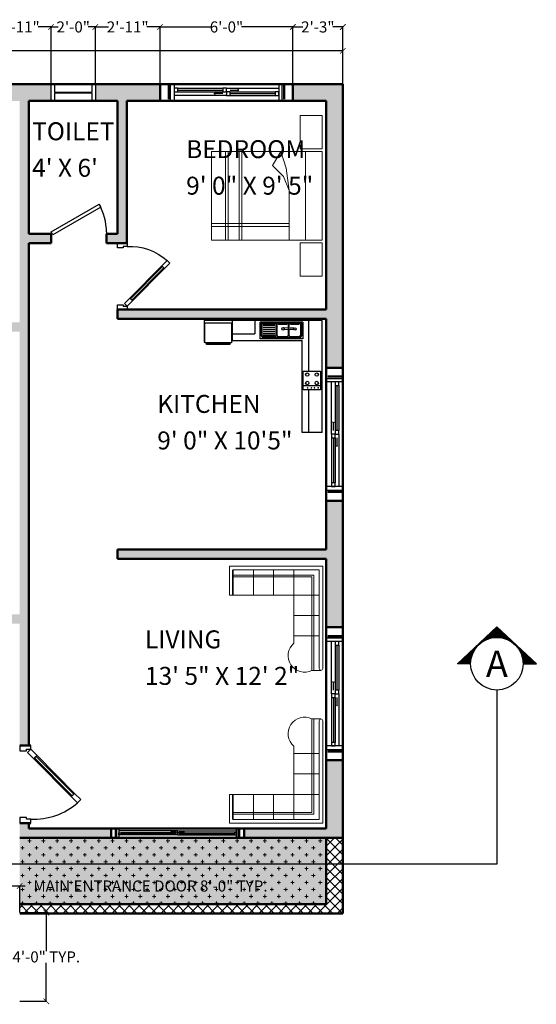
# Model space of a CAD drawing. Units: inches. Extents: x 2278 to 7495, y -71 to 1198.
# Tile 44 of 44: x 7215 to 7495, y 665 to 1198. Entities that reach past the tile are written whole.
import ezdxf
from ezdxf.enums import TextEntityAlignment as Align

# ---------------------------------------------------------------- set-up
doc = ezdxf.new("R2010")
doc.units = ezdxf.units.IN
doc.header["$MEASUREMENT"] = 0
for name, color, linetype, lineweight in [('A-ANNO-DIMS', 2, 'Continuous', 18), ('A-ANNO-SYMB', 1, 'Continuous', 25), ('A-AREA-IDEN', 3, 'Continuous', 18), ('A-Door', 3, 'Continuous', 25), ('A-FLOR-FIXT', 9, 'Continuous', 18), ('A-FURN', 8, 'Continuous', 18), ('A-Glaz', 4, 'Continuous', 25), ('A-Wall', 7, 'Continuous', 50), ('A-WALL-PATT', 8, 'Continuous', 18)]:
    doc.layers.add(name, color=color, linetype=linetype, lineweight=lineweight)
doc.layers.add('TEFRIŞ', color=11, linetype='Continuous')
doc.styles.add('KH-TRUC', font='txt', dxfattribs={"height": 200})
doc.styles.get("Standard").update_dxf_attribs({"font": 'arial.ttf'})
doc.dimstyles.get("Standard").update_dxf_attribs({"dimtxt": 6, "dimasz": 3, "dimexe": 0.18, "dimexo": 0.0625, "dimgap": 0.09, "dimtad": 0, "dimtih": 1, "dimtoh": 1, "dimdec": 0, "dimzin": 0, "dimdsep": 46, "dimlunit": 3, "dimtxsty": 'Standard', "dimblk": 'ARCHTICK', "dimcen": 0.09, "dimadec": 0, "dimazin": 0, "dimtfac": 1, "dimtdec": 0, "dimtofl": 0, "dimtmove": 0, "dimatfit": 3, "dimfxl": 1, "dimtolj": 1, "dimtzin": 0, "dimarcsym": 0})

# ---------------------------------------------------------------- blocks, each defined once
blk = doc.blocks.new('A$C1DF4181C')
blk.add_lwpolyline([(120, 128), (460.7, 466.1), (432.5, 494.5), (91.8, 156.4)], close=True)
blk.add_arc((72.4, 128.7), 593.3, 357.23132, 41.49368)
at = {"layer": 'A-Door'}
for points in [[(517.5, 522.4), (460.7, 466.1), (432.5, 494.5), (489.3, 550.8)], [(35, 100), (0, 100), (0, 0), (50, 0), (50, 50), (50, 60), (35, 60)], [(63.2, 71.6), (120, 128), (91.8, 156.4), (35, 100)], [(665, 100), (665, 60), (650, 60), (650, 50), (650, 0), (700, 0), (700, 100)]]:
    blk.add_lwpolyline(points, close=True, dxfattribs=at)
at = {"layer": 'A-Glaz'}
blk.add_lwpolyline([(112.9, 135.1), (453.6, 473.2), (439.5, 487.4), (98.8, 149.3)], close=True, dxfattribs=at)
at = {"layer": 'A-Wall'}
for p, q in [((0, 0), (0, 100)), ((0, 100), (0, 0)), ((700, 0), (700, 100)), ((700, 0), (700, 100))]:
    blk.add_line(p, q, dxfattribs=at)
blk = doc.blocks.new('*U4')
for p, q in [((0, 0), (0, -6)), ((30, 0), (30, -6))]:
    blk.add_line(p, q)
blk.add_lwpolyline([(0, 0), (25.98, 15), (26.86, 13.48), (0.87, -1.52)], close=True)
blk.add_arc((0, 0), 30, 0, 30)
blk = doc.blocks.new('BED-160')
at = {"color": 0}
for p, q in [((-0.45, 2.35), (-0.45, 2.95)), ((-0.45, 2.95), (-0.05, 2.95)), ((-0.05, 2.95), (-0.05, 2.35)), ((-0.05, 2.35), (-0.45, 2.35)), ((-2.05, 2.3), (-0.05, 2.3)), ((-2.05, 0.7), (-2.05, 2.3)), ((-1.8, 0.7), (-1.8, 2.3)), ((-1.75, 0.7), (-1.75, 2.3)), ((-1.55, 0.7), (-1.55, 2.3)), ((-1.5, 0.7), (-1.5, 2.3)), ((-0.8, 2.3), (-0.95, 2.05)), ((-0.8, 2.3), (-0.7, 2)), ((-0.35, 0.7), (-0.35, 2.3)), ((-0.05, 2.3), (-0.05, 0.7)), ((-0.95, 2.05), (-0.75, 1.85)), ((-0.7, 2), (-0.65, 1.6)), ((-0.75, 1.85), (-0.65, 1.6)), ((-0.65, 1.6), (-0.65, 0.7)), ((-0.65, 1), (-2.05, 1)), ((-0.65, 0.95), (-2.05, 0.95)), ((-0.05, 0.7), (-2.05, 0.7)), ((-0.45, 0.65), (-0.05, 0.65)), ((-0.45, 0.05), (-0.45, 0.65)), ((-0.05, 0.65), (-0.05, 0.05)), ((-0.05, 0.05), (-0.45, 0.05))]:
    blk.add_line(p, q, dxfattribs=at)
blk = doc.blocks.new('A$C008029BD')
at = {"layer": 'TEFRIŞ', "ltscale": 0.05}
for p, q in [((0, 0), (0, -3.55)), ((3.37, 0), (0, 0)), ((3.37, 0), (3.37, -0.6)), ((1.522, -0.4), (0, -0.4)), ((0.05, -0.581), (0.05, -1.869)), ((0.05, -0.581), (0.55, -0.581)), ((0.55, -0.581), (0.55, -1.869)), ((3.37, -0.4), (2.083, -0.4)), ((0.086, -1.773), (0.086, -0.677)), ((0.096, -0.617), (0.454, -0.617)), ((0.099, -0.659), (0.457, -0.659)), ((0.113, -0.954), (0.113, -0.695)), ((0.23, -0.846), (0.229, -0.967)), ((0.28, -0.846), (0.277, -1.158)), ((0.493, -0.695), (0.493, -0.954)), ((0.514, -0.677), (0.514, -1.773)), ((0.6, -2.71), (0.6, -0.6)), ((3.37, -0.6), (0.6, -0.6)), ((0.096, -1.024), (0.454, -1.024)), ((0.457, -0.99), (0.099, -0.99)), ((0.11, -1.319), (0.11, -1.06)), ((0.228, -1.02), (0.227, -1.159)), ((0.49, -1.06), (0.49, -1.319)), ((0.454, -1.355), (0.096, -1.355)), ((0.096, -1.391), (0.454, -1.391)), ((0.11, -1.773), (0.11, -1.427)), ((0.154, -1.773), (0.154, -1.427)), ((0.214, -1.773), (0.214, -1.427)), ((0.274, -1.773), (0.274, -1.427)), ((0.334, -1.773), (0.334, -1.427)), ((0.39, -1.773), (0.39, -1.427)), ((0.444, -1.773), (0.444, -1.427)), ((0.49, -1.427), (0.49, -1.773)), ((0, -2.025), (0.4, -2.025)), ((0.55, -1.869), (0.05, -1.869)), ((0.454, -1.809), (0.096, -1.809)), ((0.454, -1.833), (0.096, -1.833)), ((0.4, -2.71), (0.4, -2.025)), ((0, -2.71), (0.6, -2.71)), ((0, -3.55), (0.65, -3.55))]:
    blk.add_line(p, q, dxfattribs=at)
at = {"layer": 'TEFRIŞ'}
blk.add_line((1.969, -0.05), (1.969, -0.572), dxfattribs=at)
at = {"layer": 'TEFRIŞ', "ltscale": 0.05}
for points in [[(1.522, -0.05), (2.083, -0.05), (2.083, -0.572), (1.522, -0.572)], [(0.67, -2.73), (0.67, -3.53), (0.07, -3.53), (0.07, -2.73)], [(0.72, -2.78), (0.72, -3.48), (0.67, -3.48), (0.67, -2.78)]]:
    blk.add_lwpolyline(points, close=True, dxfattribs=at)
at = {"layer": 'TEFRIŞ', "const_width": 0.025}
for points in [[(2.014, -0.123, 1), (2.039, -0.123, 1)], [(2.014, -0.236, 1), (2.039, -0.236, 1)], [(2.014, -0.327, 1), (2.039, -0.327, 1)], [(2.014, -0.44, 1), (2.039, -0.44, 1)]]:
    blk.add_lwpolyline(points, format="xyb", close=True, dxfattribs=at)
at = {"layer": 'TEFRIŞ', "ltscale": 0.05}
for centre, radius in [((1.628, -0.164), 0.0505), ((1.628, -0.45), 0.0505), ((0.255, -0.82), 0.036), ((0.252, -1.184), 0.036)]:
    blk.add_circle(centre, radius, dxfattribs=at)
at = {"layer": 'TEFRIŞ'}
for centre in [(1.88, -0.164), (1.88, -0.45)]:
    blk.add_circle(centre, 0.0505, dxfattribs=at)
at = {"layer": 'TEFRIŞ', "ltscale": 0.05}
for centre, radius, start, end in [((0.108, -0.649), 0.0351, 110.4976, 230.5777), ((0.118, -0.673), 0.023, 143.9853, 258.5157), ((0.454, -0.677), 0.06, 0, 90), ((0.457, -0.695), 0.036, 0, 90), ((0.115, -1.038), 0.023, 143.9853, 258.5157), ((0.118, -0.976), 0.023, 101.4843, 216.0147), ((0.454, -1.06), 0.036, 0, 90), ((0.457, -0.954), 0.036, 270, 0), ((0.115, -1.341), 0.023, 101.4843, 216.0147), ((0.115, -1.405), 0.023, 143.9853, 258.5157), ((0.454, -1.319), 0.036, 270, 0), ((0.454, -1.427), 0.036, 0, 90), ((0.108, -1.801), 0.0351, 129.4223, 249.5024), ((0.115, -1.796), 0.023, 101.4843, 216.0147), ((0.454, -1.773), 0.06, 270, 0), ((0.454, -1.773), 0.036, 270, 0)]:
    blk.add_arc(centre, radius, start, end, dxfattribs=at)
blk = doc.blocks.new('_ArchTick')
at = {"color": 0, "linetype": 'ByBlock', "const_width": 0.15}
blk.add_lwpolyline([(-0.5, -0.5), (0.5, 0.5)], dxfattribs=at)
blk = doc.blocks.new('*D28')
at = {"layer": 'A-ANNO-DIMS', "color": 0, "lineweight": -2, "transparency": 16777216}
for p, q in [((6987.12, 1163.53), (6987.12, 1181.72)), ((6987.12, 1181.54), (7178.22, 1181.54)), ((7390.12, 1181.54), (7199.01, 1181.54)), ((7390.12, 1163.53), (7390.12, 1181.72))]:
    blk.add_line(p, q, dxfattribs=at)
at = {"layer": 'Defpoints', "color": 0, "transparency": 16777216}
for p in [(7390.12, 1181.54), (6987.12, 1163.47), (7390.12, 1163.47)]:
    blk.add_point(p, dxfattribs=at)
at = {"layer": 'A-ANNO-DIMS', "color": 0, "lineweight": -2, "transparency": 16777216, "xscale": 3, "yscale": 3, "zscale": 3, "rotation": 180}
blk.add_blockref('_ArchTick', (6987.12, 1181.54), dxfattribs=at)
at = {"layer": 'A-ANNO-DIMS', "color": 0, "lineweight": -2, "transparency": 16777216, "xscale": 3, "yscale": 3, "zscale": 3}
blk.add_blockref('_ArchTick', (7390.12, 1181.54), dxfattribs=at)
at = {"layer": 'A-ANNO-DIMS', "color": 0, "transparency": 16777216, "insert": (7188.62, 1181.54), "char_height": 6, "attachment_point": 5}
blk.add_mtext('\\A1;33\'-7"', dxfattribs=at)
blk = doc.blocks.new('*X31')
at = {"color": 0}
for p, q in [((19.68, 20.47), (19.71, 20.51)), ((19.68, 20.38), (19.76, 20.46)), ((19.68, 20.29), (19.8, 20.42)), ((19.68, 20.21), (19.84, 20.37)), ((19.68, 20.12), (19.88, 20.33)), ((19.68, 20.03), (19.93, 20.28)), ((19.68, 19.94), (19.97, 20.23)), ((19.68, 19.85), (20.01, 20.19)), ((19.68, 19.76), (20.05, 20.14)), ((19.68, 19.68), (20.1, 20.1)), ((19.68, 19.59), (20.14, 20.05)), ((19.68, 19.5), (20.18, 20.01)), ((19.68, 19.41), (20.22, 19.96)), ((19.68, 19.32), (20.27, 19.91)), ((19.68, 19.23), (20.31, 19.87)), ((19.68, 19.15), (20.35, 19.82)), ((19.68, 19.06), (20.4, 19.78)), ((19.68, 18.97), (20.44, 19.73)), ((19.68, 18.88), (20.48, 19.69)), ((19.68, 18.79), (20.52, 19.64)), ((19.68, 18.7), (20.57, 19.59)), ((19.68, 18.62), (20.61, 19.55)), ((19.68, 18.53), (20.65, 19.5)), ((19.68, 18.44), (20.69, 19.46)), ((19.68, 18.35), (20.74, 19.41)), ((19.68, 18.26), (20.78, 19.37)), ((19.68, 18.17), (20.82, 19.32)), ((19.68, 18.08), (20.86, 19.27)), ((19.73, 18.05), (20.91, 19.23)), ((19.81, 18.05), (20.95, 19.18)), ((19.9, 18.04), (20.99, 19.14)), ((19.98, 18.04), (21.04, 19.09)), ((20.06, 18.03), (21.08, 19.05)), ((20.15, 18.03), (21.12, 19)), ((20.23, 18.02), (21.16, 18.95)), ((20.31, 18.01), (21.21, 18.91)), ((20.38, 18), (21.25, 18.86)), ((20.46, 17.99), (21.29, 18.82)), ((20.54, 17.97), (21.33, 18.77)), ((20.61, 17.96), (21.38, 18.73)), ((20.68, 17.94), (21.42, 18.68)), ((20.76, 17.93), (21.46, 18.63)), ((20.83, 17.91), (21.5, 18.59)), ((20.9, 17.9), (21.55, 18.54)), ((20.97, 17.88), (21.59, 18.5)), ((21.04, 17.86), (21.63, 18.45)), ((21.11, 17.84), (21.68, 18.41)), ((21.18, 17.82), (21.72, 18.36)), ((21.24, 17.8), (21.76, 18.31)), ((21.31, 17.77), (21.8, 18.27)), ((21.37, 17.75), (21.85, 18.22)), ((21.44, 17.73), (21.89, 18.18)), ((21.5, 17.7), (21.93, 18.13)), ((21.57, 17.68), (21.97, 18.08)), ((21.63, 17.65), (22.02, 18.04)), ((21.69, 17.62), (22.06, 17.99)), ((21.75, 17.6), (22.1, 17.95)), ((21.81, 17.57), (22.14, 17.9)), ((21.87, 17.54), (22.19, 17.86)), ((21.93, 17.51), (22.23, 17.81)), ((21.99, 17.48), (22.27, 17.76)), ((22.05, 17.45), (22.32, 17.72)), ((22.1, 17.42), (22.36, 17.67)), ((22.16, 17.39), (22.4, 17.63)), ((22.22, 17.35), (22.44, 17.58)), ((22.27, 17.32), (22.49, 17.54)), ((22.33, 17.29), (22.53, 17.49)), ((22.38, 17.25), (22.57, 17.44)), ((22.43, 17.22), (22.61, 17.4)), ((22.49, 17.18), (22.66, 17.35)), ((22.54, 17.15), (22.7, 17.31)), ((22.59, 17.11), (22.74, 17.26)), ((22.64, 17.07), (22.78, 17.22)), ((22.69, 17.04), (22.83, 17.17)), ((22.74, 17), (22.87, 17.12)), ((22.79, 16.96), (22.91, 17.08)), ((22.84, 16.92), (22.96, 17.03)), ((22.89, 16.88), (23, 16.99)), ((22.94, 16.84), (23.04, 16.94)), ((22.98, 16.8), (23.08, 16.9)), ((23.03, 16.75), (23.13, 16.85)), ((23.08, 16.71), (23.17, 16.8)), ((23.12, 16.67), (23.21, 16.76)), ((23.17, 16.63), (23.25, 16.71)), ((23.21, 16.58), (23.3, 16.67)), ((23.26, 16.54), (23.34, 16.62)), ((23.3, 16.49), (23.38, 16.58)), ((23.34, 16.45), (23.42, 16.53)), ((23.38, 16.4), (23.47, 16.48)), ((23.43, 16.35), (23.51, 16.44)), ((23.47, 16.31), (23.55, 16.39)), ((23.51, 16.26), (23.6, 16.35)), ((23.55, 16.21), (23.64, 16.3)), ((23.59, 16.16), (23.68, 16.26)), ((23.63, 16.11), (23.72, 16.21)), ((23.66, 16.06), (23.77, 16.16)), ((23.7, 16.01), (23.81, 16.12)), ((23.74, 15.96), (23.85, 16.07)), ((23.78, 15.91), (23.89, 16.03)), ((23.81, 15.86), (23.94, 15.98)), ((23.85, 15.8), (23.98, 15.94)), ((23.88, 15.75), (24.02, 15.89)), ((23.92, 15.7), (24.06, 15.84)), ((23.95, 15.64), (24.11, 15.8)), ((23.98, 15.59), (24.15, 15.75)), ((24.02, 15.53), (24.19, 15.71)), ((24.05, 15.47), (24.24, 15.66)), ((24.08, 15.42), (24.28, 15.62)), ((24.11, 15.36), (24.32, 15.57)), ((24.14, 15.3), (24.36, 15.52)), ((24.17, 15.24), (24.41, 15.48)), ((24.2, 15.18), (24.45, 15.43)), ((24.23, 15.12), (24.49, 15.39)), ((24.25, 15.06), (24.53, 15.34)), ((24.28, 15), (24.58, 15.3)), ((24.31, 14.94), (24.62, 15.25)), ((24.33, 14.87), (24.66, 15.2)), ((24.36, 14.81), (24.7, 15.16)), ((24.38, 14.74), (24.75, 15.11)), ((24.4, 14.68), (24.79, 15.07)), ((24.42, 14.61), (24.83, 15.02)), ((24.45, 14.55), (24.88, 14.98)), ((24.04, 10.6), (26.58, 13.15)), ((24.14, 10.79), (26.54, 13.19)), ((24.22, 10.96), (26.5, 13.24)), ((24.29, 11.12), (26.45, 13.28)), ((24.35, 11.27), (26.41, 13.33)), ((24.4, 11.41), (26.37, 13.38)), ((24.44, 11.54), (26.33, 13.42)), ((24.47, 14.48), (24.92, 14.93)), ((24.48, 11.66), (26.28, 13.47)), ((24.49, 14.41), (24.96, 14.88)), ((24.51, 14.34), (25, 14.84)), ((24.51, 11.79), (26.24, 13.51)), ((24.52, 14.27), (25.05, 14.79)), ((24.54, 14.2), (25.09, 14.75)), ((24.54, 11.9), (26.2, 13.56)), ((24.56, 14.13), (25.13, 14.7)), ((24.57, 14.06), (25.17, 14.66)), ((24.57, 12.02), (26.16, 13.6)), ((24.59, 13.98), (25.22, 14.61)), ((24.59, 12.13), (26.11, 13.65)), ((24.6, 13.91), (25.26, 14.56)), ((24.61, 13.83), (25.3, 14.52)), ((24.61, 12.24), (26.07, 13.7)), ((24.63, 13.75), (25.35, 14.47)), ((24.63, 12.34), (26.03, 13.74)), ((24.64, 13.68), (25.39, 14.43)), ((24.64, 12.44), (25.99, 13.79)), ((24.65, 13.6), (25.43, 14.38)), ((24.65, 13.52), (25.47, 14.34)), ((24.65, 12.54), (25.94, 13.83)), ((24.66, 13.44), (25.52, 14.29)), ((24.66, 12.64), (25.9, 13.88)), ((24.67, 13.35), (25.56, 14.24)), ((24.67, 13.27), (25.6, 14.2)), ((24.67, 13.18), (25.64, 14.15)), ((24.67, 12.92), (25.77, 14.02)), ((24.67, 12.83), (25.81, 13.97)), ((24.67, 12.73), (25.86, 13.92)), ((24.68, 13.1), (25.69, 14.11)), ((24.68, 13.01), (25.73, 14.06)), ((19.68, 5.98), (25.68, 11.98)), ((23.72, 10.11), (26.67, 13.06)), ((23.91, 10.38), (26.63, 13.1)), ((19.68, 5.89), (24.44, 10.65)), ((19.68, 5.8), (23.2, 9.32)), ((19.68, 6.06), (22.61, 9)), ((19.68, 6.15), (22.34, 8.81)), ((19.68, 6.24), (22.12, 8.69)), ((19.68, 6.33), (21.93, 8.58)), ((19.68, 6.42), (21.76, 8.5)), ((19.68, 6.51), (21.6, 8.43)), ((19.68, 6.59), (21.46, 8.37)), ((19.68, 6.68), (21.32, 8.32)), ((19.68, 6.77), (21.19, 8.28)), ((19.68, 6.86), (21.06, 8.24)), ((19.68, 6.95), (20.94, 8.21)), ((19.68, 7.04), (20.82, 8.18)), ((19.68, 7.12), (20.71, 8.15)), ((19.68, 7.21), (20.6, 8.13)), ((19.68, 7.3), (20.49, 8.11)), ((19.68, 7.39), (20.38, 8.1)), ((19.68, 7.48), (20.28, 8.08)), ((19.68, 7.57), (20.18, 8.07)), ((19.68, 7.74), (19.99, 8.06)), ((19.68, 7.66), (20.08, 8.06)), ((19.68, 8.01), (19.71, 8.05)), ((19.68, 7.92), (19.8, 8.05)), ((19.68, 7.83), (19.9, 8.05)), ((19.68, 5.71), (21.96, 8)), ((19.68, 5.62), (20.73, 6.67))]:
    blk.add_line(p, q, dxfattribs=at)
blk = doc.blocks.new('A$C695C76AC')
for p, q in [((5.36, 5), (12.86, 12)), ((20.36, 5), (12.86, 12)), ((7.86, 5), (5.36, 5)), ((17.86, 5), (20.36, 5))]:
    blk.add_line(p, q)
blk.add_circle((12.86, 5), 5)
at = {"rotation": 90}
blk.add_blockref('*X31', (25.9, -14.68), dxfattribs=at)
at = {"style": 'KH-TRUC'}
blk.add_attdef('KH-MC', text='', height=5, dxfattribs=at).set_placement((12.86, 5), align=Align.MIDDLE_CENTER)
blk = doc.blocks.new('*D55')
at = {"layer": 'A-ANNO-DIMS', "color": 0, "lineweight": -2, "transparency": 16777216}
for p, q in [((7119.12, 715.03), (7119.12, 729.55)), ((7119.12, 729.37), (7215.12, 729.37)), ((7215.12, 715.03), (7215.12, 729.55)), ((7215.12, 729.37), (7218.12, 729.37))]:
    blk.add_line(p, q, dxfattribs=at)
at = {"layer": 'Defpoints', "color": 0, "transparency": 16777216}
for p in [(7215.12, 729.37), (7119.12, 714.97), (7215.12, 714.97)]:
    blk.add_point(p, dxfattribs=at)
at = {"layer": 'A-ANNO-DIMS', "color": 0, "lineweight": -2, "transparency": 16777216, "xscale": 3, "yscale": 3, "zscale": 3, "rotation": 180}
blk.add_blockref('_ArchTick', (7119.12, 729.37), dxfattribs=at)
at = {"layer": 'A-ANNO-DIMS', "color": 0, "lineweight": -2, "transparency": 16777216, "xscale": 3, "yscale": 3, "zscale": 3}
blk.add_blockref('_ArchTick', (7215.12, 729.37), dxfattribs=at)
at = {"layer": 'A-ANNO-DIMS', "color": 0, "transparency": 16777216, "insert": (7285.95, 729.37), "char_height": 6, "attachment_point": 5}
blk.add_mtext('\\A1;MAIN ENTRANCE DOOR 8\'-0" TYP.', dxfattribs=at)
blk = doc.blocks.new('*D56')
at = {"layer": 'A-ANNO-DIMS', "color": 0, "lineweight": -2, "transparency": 16777216}
for p, q in [((7215.18, 714.97), (7229.7, 714.97)), ((7229.52, 714.97), (7229.52, 694.12)), ((7229.52, 666.97), (7229.52, 687.81)), ((7215.18, 666.97), (7229.7, 666.97))]:
    blk.add_line(p, q, dxfattribs=at)
at = {"layer": 'Defpoints', "color": 0, "transparency": 16777216}
for p in [(7215.12, 714.97), (7215.12, 666.97), (7229.52, 666.97)]:
    blk.add_point(p, dxfattribs=at)
at = {"layer": 'A-ANNO-DIMS', "color": 0, "lineweight": -2, "transparency": 16777216, "xscale": 3, "yscale": 3, "zscale": 3}
for p, rotation in [((7229.52, 714.97), 90), ((7229.52, 666.97), 270)]:
    blk.add_blockref('_ArchTick', p, dxfattribs=dict(at, rotation=rotation))
at = {"layer": 'A-ANNO-DIMS', "color": 0, "transparency": 16777216, "insert": (7229.52, 690.97), "char_height": 6, "attachment_point": 5}
blk.add_mtext('\\A1;4\'-0" TYP.', dxfattribs=at)
blk = doc.blocks.new('*D97')
at = {"layer": 'A-ANNO-DIMS', "color": 0, "lineweight": -2, "transparency": 16777216}
for p, q in [((7197.12, 1163.53), (7197.12, 1194.65)), ((7197.12, 1194.47), (7204.17, 1194.47)), ((7232.12, 1194.47), (7225.06, 1194.47)), ((7232.12, 1163.53), (7232.12, 1194.65))]:
    blk.add_line(p, q, dxfattribs=at)
at = {"layer": 'Defpoints', "color": 0, "transparency": 16777216}
for p in [(7232.12, 1194.47), (7197.12, 1163.47), (7232.12, 1163.47)]:
    blk.add_point(p, dxfattribs=at)
at = {"layer": 'A-ANNO-DIMS', "color": 0, "lineweight": -2, "transparency": 16777216, "xscale": 3, "yscale": 3, "zscale": 3, "rotation": 180}
blk.add_blockref('_ArchTick', (7197.12, 1194.47), dxfattribs=at)
at = {"layer": 'A-ANNO-DIMS', "color": 0, "lineweight": -2, "transparency": 16777216, "xscale": 3, "yscale": 3, "zscale": 3}
blk.add_blockref('_ArchTick', (7232.12, 1194.47), dxfattribs=at)
at = {"layer": 'A-ANNO-DIMS', "color": 0, "transparency": 16777216, "insert": (7214.62, 1194.47), "char_height": 6, "attachment_point": 5}
blk.add_mtext('\\A1;2\'-11"', dxfattribs=at)
blk = doc.blocks.new('*D98')
at = {"layer": 'A-ANNO-DIMS', "color": 0, "lineweight": -2, "transparency": 16777216}
for p, q in [((7232.12, 1163.53), (7232.12, 1194.65)), ((7232.12, 1194.47), (7236, 1194.47)), ((7256.12, 1194.47), (7252.23, 1194.47)), ((7256.12, 1163.53), (7256.12, 1194.65))]:
    blk.add_line(p, q, dxfattribs=at)
at = {"layer": 'Defpoints', "color": 0, "transparency": 16777216}
for p in [(7256.12, 1194.47), (7232.12, 1163.47), (7256.12, 1163.47)]:
    blk.add_point(p, dxfattribs=at)
at = {"layer": 'A-ANNO-DIMS', "color": 0, "lineweight": -2, "transparency": 16777216, "xscale": 3, "yscale": 3, "zscale": 3, "rotation": 180}
blk.add_blockref('_ArchTick', (7232.12, 1194.47), dxfattribs=at)
at = {"layer": 'A-ANNO-DIMS', "color": 0, "lineweight": -2, "transparency": 16777216, "xscale": 3, "yscale": 3, "zscale": 3}
blk.add_blockref('_ArchTick', (7256.12, 1194.47), dxfattribs=at)
at = {"layer": 'A-ANNO-DIMS', "color": 0, "transparency": 16777216, "insert": (7244.12, 1194.47), "char_height": 6, "attachment_point": 5}
blk.add_mtext('\\A1;2\'-0"', dxfattribs=at)
blk = doc.blocks.new('*D99')
at = {"layer": 'A-ANNO-DIMS', "color": 0, "lineweight": -2, "transparency": 16777216}
for p, q in [((7256.12, 1163.53), (7256.12, 1194.65)), ((7256.12, 1194.47), (7263.17, 1194.47)), ((7291.12, 1194.47), (7284.06, 1194.47)), ((7291.12, 1163.53), (7291.12, 1194.65))]:
    blk.add_line(p, q, dxfattribs=at)
at = {"layer": 'Defpoints', "color": 0, "transparency": 16777216}
for p in [(7291.12, 1194.47), (7256.12, 1163.47), (7291.12, 1163.47)]:
    blk.add_point(p, dxfattribs=at)
at = {"layer": 'A-ANNO-DIMS', "color": 0, "lineweight": -2, "transparency": 16777216, "xscale": 3, "yscale": 3, "zscale": 3, "rotation": 180}
blk.add_blockref('_ArchTick', (7256.12, 1194.47), dxfattribs=at)
at = {"layer": 'A-ANNO-DIMS', "color": 0, "lineweight": -2, "transparency": 16777216, "xscale": 3, "yscale": 3, "zscale": 3}
blk.add_blockref('_ArchTick', (7291.12, 1194.47), dxfattribs=at)
at = {"layer": 'A-ANNO-DIMS', "color": 0, "transparency": 16777216, "insert": (7273.62, 1194.47), "char_height": 6, "attachment_point": 5}
blk.add_mtext('\\A1;2\'-11"', dxfattribs=at)
blk = doc.blocks.new('*D100')
at = {"layer": 'A-ANNO-DIMS', "color": 0, "lineweight": -2, "transparency": 16777216}
for p, q in [((7291.12, 1163.53), (7291.12, 1194.65)), ((7291.12, 1194.47), (7319.03, 1194.47)), ((7363.12, 1194.47), (7335.2, 1194.47)), ((7363.12, 1163.53), (7363.12, 1194.65))]:
    blk.add_line(p, q, dxfattribs=at)
at = {"layer": 'Defpoints', "color": 0, "transparency": 16777216}
for p in [(7363.12, 1194.47), (7291.12, 1163.47), (7363.12, 1163.47)]:
    blk.add_point(p, dxfattribs=at)
at = {"layer": 'A-ANNO-DIMS', "color": 0, "lineweight": -2, "transparency": 16777216, "xscale": 3, "yscale": 3, "zscale": 3, "rotation": 180}
blk.add_blockref('_ArchTick', (7291.12, 1194.47), dxfattribs=at)
at = {"layer": 'A-ANNO-DIMS', "color": 0, "lineweight": -2, "transparency": 16777216, "xscale": 3, "yscale": 3, "zscale": 3}
blk.add_blockref('_ArchTick', (7363.12, 1194.47), dxfattribs=at)
at = {"layer": 'A-ANNO-DIMS', "color": 0, "transparency": 16777216, "insert": (7327.12, 1194.47), "char_height": 6, "attachment_point": 5}
blk.add_mtext('\\A1;6\'-0"', dxfattribs=at)
blk = doc.blocks.new('*D101')
at = {"layer": 'A-ANNO-DIMS', "color": 0, "lineweight": -2, "transparency": 16777216}
for p, q in [((7363.12, 1163.53), (7363.12, 1194.65)), ((7363.12, 1194.47), (7368.5, 1194.47)), ((7390.12, 1194.47), (7384.73, 1194.47)), ((7390.12, 1163.53), (7390.12, 1194.65))]:
    blk.add_line(p, q, dxfattribs=at)
at = {"layer": 'Defpoints', "color": 0, "transparency": 16777216}
for p in [(7390.12, 1194.47), (7363.12, 1163.47), (7390.12, 1163.47)]:
    blk.add_point(p, dxfattribs=at)
at = {"layer": 'A-ANNO-DIMS', "color": 0, "lineweight": -2, "transparency": 16777216, "xscale": 3, "yscale": 3, "zscale": 3, "rotation": 180}
blk.add_blockref('_ArchTick', (7363.12, 1194.47), dxfattribs=at)
at = {"layer": 'A-ANNO-DIMS', "color": 0, "lineweight": -2, "transparency": 16777216, "xscale": 3, "yscale": 3, "zscale": 3}
blk.add_blockref('_ArchTick', (7390.12, 1194.47), dxfattribs=at)
at = {"layer": 'A-ANNO-DIMS', "color": 0, "transparency": 16777216, "insert": (7376.62, 1194.47), "char_height": 6, "attachment_point": 5}
blk.add_mtext('\\A1;2\'-3"', dxfattribs=at)

msp = doc.modelspace()

# ---------------------------------------------------------------- hatches: boundary and pattern name
at = {"layer": 'A-WALL-PATT'}
h = msp.add_hatch(dxfattribs=at)
h.set_pattern_fill('ANSI36', color=256, scale=30)
h.set_pattern_definition([(45, (4673.2453, 0), (1.988738, 7.2920387), [9.375, -1.875, 0, -1.875])])
h.paths.add_polyline_path([(7016.37, 957.47), (6996.12, 957.47), (6996.12, 1029.47), (7025.12, 1029.47), (7025.12, 1034.47), (6996.12, 1034.47), (6996.12, 1154.47), (7013.12, 1154.47), (7013.12, 1163.47), (6987.12, 1163.47), (6987.12, 710.47), (7119.12, 710.47), (7119.12, 719.47), (6996.12, 719.47), (6996.12, 807.47), (7078.12, 807.47), (7078.12, 812.47), (7066.12, 812.47), (7066.12, 881.47), (7061.12, 881.47), (7061.12, 812.47), (6996.12, 812.47), (6996.12, 911.47), (7019.12, 911.47), (7019.12, 916.47), (6996.12, 916.47), (6996.12, 952.47), (7016.37, 952.47)])
h.paths.add_polyline_path([(7125.12, 1163.47), (7085.12, 1163.47), (7085.12, 1154.47), (7102.12, 1154.47), (7102.12, 1034.47), (7102.12, 1029.47), (7107.12, 1029.47), (7107.12, 1154.47), (7125.12, 1154.47)])
h.paths.add_polyline_path([(7232.12, 1163.47), (7197.12, 1163.47), (7197.12, 1154.47), (7215.12, 1154.47), (7215.12, 1034.47), (7149.12, 1034.47), (7149.12, 1029.47), (7215.12, 1029.47), (7215.12, 943.47), (7215.12, 940.13), (7215.12, 876.47), (7167.12, 876.47), (7167.12, 943.47), (7162.12, 943.47), (7162.12, 871.47), (7162.12, 865.74), (7167.12, 865.74), (7167.12, 871.47), (7215.12, 871.47), (7215.12, 805.47), (7220.12, 805.47), (7220.12, 1077.47), (7232.12, 1077.47), (7232.12, 1082.47), (7220.12, 1082.47), (7220.12, 1154.47), (7232.12, 1154.47)])
h.paths.add_polyline_path([(7390.12, 937.97), (7381.12, 937.97), (7381.12, 911.47), (7268.12, 911.47), (7268.12, 906.47), (7381.12, 906.47), (7381.12, 869.47), (7390.12, 869.47)])
h.paths.add_polyline_path([(7390.12, 1163.47), (7363.12, 1163.47), (7363.12, 1154.47), (7381.12, 1154.47), (7381.12, 1041.47), (7268.12, 1041.47), (7268.12, 1036.47), (7381.12, 1036.47), (7381.12, 1009.97), (7390.12, 1009.97)])
h.paths.add_polyline_path([(7291.12, 1163.47), (7256.12, 1163.47), (7256.12, 1154.47), (7268.12, 1154.47), (7268.12, 1082.47), (7262.12, 1082.47), (7262.12, 1077.47), (7273.12, 1077.47), (7273.12, 1154.47), (7291.12, 1154.47)])
h.paths.add_polyline_path([(7390.12, 797.47), (7381.12, 797.47), (7381.12, 760.47), (7336.62, 760.47), (7336.62, 755.47), (7390.12, 755.47)])
h.paths.add_polyline_path([(7264.62, 760.47), (7220.12, 760.47), (7220.12, 763.47), (7215.12, 763.47), (7215.12, 755.47), (7264.62, 755.47)])
h = msp.add_hatch(dxfattribs=at)
h.set_pattern_fill('ANSI37', color=256, scale=30)
h.set_pattern_definition([(45, (4673.2453, 0), (-2.6516504, 2.6516504), []), (135, (4673.2453, 0), (-2.6516504, -2.6516504), [])])
h.paths.add_polyline_path([(7390.12, 755.47), (7381.12, 755.47), (7381.12, 719.47), (7215.12, 719.47), (7215.12, 714.47), (7390.12, 714.47)])
at = {"layer": 'A-WALL-PATT', "transparency": 33554562}
h = msp.add_hatch(color=256, dxfattribs=at)
h.dxf.hatch_style = 1
h.paths.add_polyline_path([(7381.12, 755.47), (7215.12, 755.47), (7215.12, 719.47), (7381.12, 719.47)])
h = msp.add_hatch(dxfattribs=at)
h.set_pattern_fill('CROSS', color=256, scale=15)
h.set_pattern_definition([(0, (4673.2453, 0), (3.75, 3.75), [1.875, -5.625]), (90, (4674.1828, -0.9375), (-3.75, 3.75), [1.875, -5.625])])
h.paths.add_polyline_path([(7381.12, 755.47), (7215.12, 755.47), (7215.12, 719.47), (7381.12, 719.47)])

# ---------------------------------------------------------------- linework, layer by layer
at = {"layer": 'A-ANNO-SYMB'}
for p, q in [((7473.67, 741.41), (7473.67, 835.33)), ((6942.63, 741.41), (7473.67, 741.41))]:
    msp.add_line(p, q, dxfattribs=at)
at = {"layer": 'A-FURN'}
for p, q in [((7379.26, 902.55), (7328.74, 902.55)), ((7328.74, 902.55), (7328.74, 886.91)), ((7379.26, 847.04), (7379.26, 902.55)), ((7330.37, 900.59), (7330.37, 886.91)), ((7377.31, 900.59), (7330.7, 900.59)), ((7330.7, 900.59), (7330.7, 886.91)), ((7374.37, 897.66), (7330.7, 897.66)), ((7373.4, 896.68), (7330.7, 896.68)), ((7341.78, 900.59), (7341.78, 886.91)), ((7352.54, 900.59), (7352.54, 886.91)), ((7363.62, 900.59), (7363.62, 864.74)), ((7373.4, 846.06), (7373.4, 896.68)), ((7374.37, 846.06), (7374.37, 897.66)), ((7377.31, 847.04), (7377.31, 900.59)), ((7328.74, 886.91), (7377.31, 886.91)), ((7363.62, 889.51), (7363.62, 864.74)), ((7363.62, 875.82), (7377.31, 875.82)), ((7363.62, 864.74), (7377.31, 864.74)), ((7363.62, 864.74), (7377.31, 864.74)), ((7363.62, 864.74), (7363.62, 860.83)), ((7378.29, 846.06), (7373.4, 846.06)), ((7373.4, 819.82), (7373.4, 769.19)), ((7378.29, 819.82), (7373.4, 819.82)), ((7374.37, 819.82), (7374.37, 768.22)), ((7377.31, 818.84), (7377.31, 765.28)), ((7379.26, 818.84), (7379.26, 763.33)), ((7363.62, 801.14), (7363.62, 805.05)), ((7363.62, 765.28), (7363.62, 801.14)), ((7363.62, 776.37), (7363.62, 801.14)), ((7363.62, 801.14), (7377.31, 801.14)), ((7363.62, 801.14), (7377.31, 801.14)), ((7363.62, 790.05), (7377.31, 790.05)), ((7328.74, 778.97), (7377.31, 778.97)), ((7328.74, 763.33), (7328.74, 778.97)), ((7330.37, 765.28), (7330.37, 778.97)), ((7330.7, 765.28), (7330.7, 778.97)), ((7341.78, 765.28), (7341.78, 778.97)), ((7352.54, 765.28), (7352.54, 778.97)), ((7373.4, 769.19), (7330.7, 769.19)), ((7374.37, 768.22), (7330.7, 768.22)), ((7379.26, 763.33), (7328.74, 763.33)), ((7377.31, 765.28), (7330.7, 765.28))]:
    msp.add_line(p, q, dxfattribs=at)
for centre, radius, start, end in [((7369.43, 854.05), 8.93, 130.6021, 296.4078), ((7378.29, 847.04), 0.978, 180, 0), ((7369.43, 811.82), 8.93, 63.5922, 229.3979), ((7378.29, 818.84), 0.978, 0, 180)]:
    msp.add_arc(centre, radius, start, end, dxfattribs=at)
at = {"layer": 'A-Glaz'}
for p, q in [((7232.12, 1163.47), (7256.12, 1163.47)), ((7232.12, 1154.47), (7232.12, 1163.47)), ((7234.12, 1159.17), (7234.12, 1163.47)), ((7254.12, 1163.47), (7254.12, 1159.17)), ((7256.12, 1163.47), (7256.12, 1154.47)), ((7298.82, 1163.47), (7355.41, 1163.47)), ((7234.12, 1159.17), (7254.12, 1159.17)), ((7234.12, 1154.47), (7234.12, 1158.77)), ((7234.12, 1158.77), (7254.12, 1158.77)), ((7254.12, 1158.77), (7254.12, 1154.47)), ((7327.12, 1157.39), (7298.82, 1157.39)), ((7300.77, 1161.3), (7325.16, 1161.3)), ((7300.77, 1160.32), (7325.16, 1160.32)), ((7300.77, 1159.35), (7325.16, 1159.35)), ((7325.16, 1158.37), (7320.97, 1158.37)), ((7327.12, 1161.3), (7355.41, 1161.3)), ((7329.07, 1160.32), (7333.26, 1160.32)), ((7329.07, 1159.35), (7353.46, 1159.35)), ((7329.07, 1158.37), (7353.46, 1158.37)), ((7329.07, 1157.39), (7353.46, 1157.39)), ((7256.12, 1154.47), (7232.12, 1154.47)), ((7298.82, 1154.47), (7355.41, 1154.47)), ((7381.12, 1002.27), (7381.12, 945.67)), ((7384.04, 973.97), (7384.04, 1002.27)), ((7390.12, 1002.27), (7390.12, 945.67)), ((7385.99, 1000.31), (7385.99, 975.92)), ((7386.97, 1000.31), (7386.97, 975.92)), ((7387.95, 1000.31), (7387.95, 975.92)), ((7385.02, 975.92), (7385.02, 980.11)), ((7384.04, 972.01), (7384.04, 947.62)), ((7385.02, 972.01), (7385.02, 947.62)), ((7385.99, 972.01), (7385.99, 947.62)), ((7386.97, 972.01), (7386.97, 967.82)), ((7387.95, 973.97), (7387.95, 945.67)), ((7381.12, 861.77), (7381.12, 805.17)), ((7384.04, 833.47), (7384.04, 861.77)), ((7385.99, 859.81), (7385.99, 835.42)), ((7386.97, 859.81), (7386.97, 835.42)), ((7387.95, 859.81), (7387.95, 835.42)), ((7390.12, 861.77), (7390.12, 805.17)), ((7385.02, 835.42), (7385.02, 839.61)), ((7387.95, 833.47), (7387.95, 805.17)), ((7384.04, 831.51), (7384.04, 807.12)), ((7385.02, 831.51), (7385.02, 807.12)), ((7385.99, 831.51), (7385.99, 807.12)), ((7386.97, 831.51), (7386.97, 827.32)), ((7300.62, 760.47), (7268.89, 760.47)), ((7300.62, 759.26), (7268.89, 759.26)), ((7299.53, 758.18), (7269.98, 758.18)), ((7299.53, 757.64), (7269.98, 757.64)), ((7299.53, 757.09), (7269.98, 757.09)), ((7299.53, 758.72), (7297.2, 758.72)), ((7300.62, 760.47), (7332.34, 760.47)), ((7300.62, 759.26), (7332.34, 759.26)), ((7301.7, 758.72), (7304.03, 758.72)), ((7301.7, 758.18), (7331.25, 758.18)), ((7301.7, 757.64), (7331.25, 757.64)), ((7301.7, 757.09), (7331.25, 757.09)), ((7300.62, 755.47), (7268.89, 755.47)), ((7300.62, 755.47), (7332.34, 755.47))]:
    msp.add_line(p, q, dxfattribs=at)
for points in [[(7298.82, 1154.47), (7296.86, 1154.47), (7296.86, 1163.47), (7298.82, 1163.47)], [(7355.41, 1154.47), (7357.37, 1154.47), (7357.37, 1163.47), (7355.41, 1163.47)], [(7298.82, 1159.35), (7300.77, 1159.35), (7300.77, 1161.3), (7298.82, 1161.3)], [(7320.47, 1158.37), (7320.97, 1158.66), (7320.97, 1158.08)], [(7325.16, 1159.35), (7327.12, 1159.35), (7327.12, 1161.3), (7325.16, 1161.3)], [(7327.12, 1157.39), (7329.07, 1157.39), (7329.07, 1159.35), (7327.12, 1159.35)], [(7333.76, 1160.32), (7333.26, 1160.61), (7333.26, 1160.03)], [(7353.46, 1157.39), (7355.41, 1157.39), (7355.41, 1159.35), (7353.46, 1159.35)], [(7381.12, 1002.27), (7381.12, 1004.22), (7390.12, 1004.22), (7390.12, 1002.27)], [(7385.99, 1002.27), (7385.99, 1000.31), (7387.95, 1000.31), (7387.95, 1002.27)], [(7385.02, 980.62), (7385.31, 980.11), (7384.73, 980.11)], [(7385.99, 975.92), (7385.99, 973.97), (7387.95, 973.97), (7387.95, 975.92)], [(7384.04, 973.97), (7384.04, 972.01), (7385.99, 972.01), (7385.99, 973.97)], [(7386.97, 967.32), (7387.26, 967.82), (7386.68, 967.82)], [(7381.12, 945.67), (7381.12, 943.72), (7390.12, 943.72), (7390.12, 945.67)], [(7384.04, 947.62), (7384.04, 945.67), (7385.99, 945.67), (7385.99, 947.62)], [(7381.12, 861.77), (7381.12, 863.72), (7390.12, 863.72), (7390.12, 861.77)], [(7385.99, 861.77), (7385.99, 859.81), (7387.95, 859.81), (7387.95, 861.77)], [(7385.02, 840.12), (7385.31, 839.61), (7384.73, 839.61)], [(7384.04, 833.47), (7384.04, 831.51), (7385.99, 831.51), (7385.99, 833.47)], [(7385.99, 835.42), (7385.99, 833.47), (7387.95, 833.47), (7387.95, 835.42)], [(7386.97, 826.82), (7387.26, 827.32), (7386.68, 827.32)], [(7381.12, 805.17), (7381.12, 803.22), (7390.12, 803.22), (7390.12, 805.17)], [(7384.04, 807.12), (7384.04, 805.17), (7385.99, 805.17), (7385.99, 807.12)], [(7268.89, 755.47), (7267.81, 755.47), (7267.81, 760.47), (7268.89, 760.47)], [(7269.98, 757.09), (7268.89, 757.09), (7268.89, 758.18), (7269.98, 758.18)], [(7296.92, 758.72), (7297.2, 758.88), (7297.2, 758.56)], [(7299.53, 758.18), (7300.62, 758.18), (7300.62, 759.26), (7299.53, 759.26)], [(7300.62, 757.09), (7299.53, 757.09), (7299.53, 758.18), (7300.62, 758.18)], [(7301.7, 758.18), (7300.62, 758.18), (7300.62, 759.26), (7301.7, 759.26)], [(7300.62, 757.09), (7301.7, 757.09), (7301.7, 758.18), (7300.62, 758.18)], [(7304.31, 758.72), (7304.03, 758.88), (7304.03, 758.56)], [(7331.25, 757.09), (7332.34, 757.09), (7332.34, 758.18), (7331.25, 758.18)], [(7332.34, 755.47), (7333.42, 755.47), (7333.42, 760.47), (7332.34, 760.47)]]:
    msp.add_lwpolyline(points, close=True, dxfattribs=at)
at = {"layer": 'A-Wall'}
for p, q in [((6987.12, 1163.47), (7390.12, 1163.47)), ((7291.12, 1154.47), (7291.12, 1163.47)), ((7296.86, 1163.47), (7291.12, 1163.47)), ((7295.89, 1163.25), (7295.89, 1155.44)), ((7357.37, 1163.47), (7363.12, 1163.47)), ((7358.34, 1163.25), (7358.34, 1155.44)), ((7363.12, 1154.47), (7363.12, 1163.47)), ((7390.12, 1163.47), (7390.12, 714.47)), ((7220.12, 1154.47), (7220.12, 1082.47)), ((7220.12, 1154.47), (7268.12, 1154.47)), ((7268.12, 1154.47), (7268.12, 1082.47)), ((7273.12, 1154.47), (7273.12, 1077.47)), ((7273.12, 1154.47), (7381.12, 1154.47)), ((7296.86, 1154.47), (7291.12, 1154.47)), ((7357.37, 1154.47), (7363.12, 1154.47)), ((7381.12, 1154.47), (7381.12, 1041.47)), ((7220.12, 1082.47), (7232.12, 1082.47)), ((7232.12, 1077.47), (7232.12, 1082.47)), ((7262.12, 1082.47), (7268.12, 1082.47)), ((7262.12, 1077.47), (7262.12, 1082.47)), ((7220.12, 1077.47), (7220.12, 805.47)), ((7220.12, 1077.47), (7232.12, 1077.47)), ((7262.12, 1077.47), (7273.12, 1077.47)), ((7268.12, 1041.47), (7268.12, 1036.47)), ((7268.12, 1041.47), (7381.12, 1041.47)), ((7268.12, 1036.47), (7381.12, 1036.47)), ((7381.12, 1036.47), (7381.12, 911.47)), ((7381.12, 1009.97), (7390.12, 1009.97)), ((7381.12, 1004.22), (7381.12, 1009.97)), ((7390.12, 1004.22), (7390.12, 1009.97)), ((7389.9, 1005.19), (7382.09, 1005.19)), ((7381.12, 943.72), (7381.12, 937.97)), ((7390.12, 943.72), (7390.12, 937.97)), ((7389.9, 942.74), (7382.09, 942.74)), ((7381.12, 937.97), (7390.12, 937.97)), ((7268.12, 911.47), (7381.12, 911.47)), ((7268.12, 906.47), (7268.12, 911.47)), ((7268.12, 906.47), (7381.12, 906.47)), ((7381.12, 906.47), (7381.12, 760.47)), ((7381.12, 869.47), (7390.12, 869.47)), ((7381.12, 863.72), (7381.12, 869.47)), ((7390.12, 863.72), (7390.12, 869.47)), ((7389.9, 864.69), (7382.09, 864.69)), ((7220.12, 805.47), (7215.12, 805.47)), ((7381.12, 803.22), (7381.12, 797.47)), ((7389.9, 802.24), (7382.09, 802.24)), ((7390.12, 803.22), (7390.12, 797.47)), ((7381.12, 797.47), (7390.12, 797.47)), ((7220.12, 763.47), (7215.12, 763.47)), ((7220.12, 763.47), (7220.12, 760.47)), ((7220.12, 760.47), (7381.12, 760.47)), ((7264.62, 755.47), (7264.62, 760.47)), ((7267.81, 760.47), (7264.62, 760.47)), ((7267.27, 760.35), (7267.27, 756.01)), ((7333.42, 760.47), (7336.62, 760.47)), ((7333.96, 760.35), (7333.96, 756.01)), ((7336.62, 755.47), (7336.62, 760.47)), ((7215.12, 755.47), (7390.12, 755.47)), ((7267.81, 755.47), (7264.62, 755.47)), ((7333.42, 755.47), (7336.62, 755.47)), ((7381.12, 755.47), (7381.12, 719.47)), ((7215.12, 719.47), (7381.12, 719.47)), ((7215.12, 714.47), (7390.12, 714.47))]:
    msp.add_line(p, q, dxfattribs=at)

# ---------------------------------------------------------------- block references
at = {"layer": 'A-ANNO-SYMB'}
ref = msp.add_blockref('A$C695C76AC', (7436.97, 835.47), dxfattribs=dict(at, xscale=2.847836231539501, yscale=2.847836231539501, zscale=2.847836231539501))
ref.add_attrib('KH-MC', 'A', dxfattribs={"layer": '0', "color": 3, "height": 14.24, "style": 'KH-TRUC'}).set_placement((7473.58, 849.71), align=Align.MIDDLE_CENTER)
at = {"layer": 'A-Door'}
msp.add_blockref('*U4', (7232.12, 1083.47), dxfattribs=at)
at = {"layer": 'A-Door', "rotation": 270}
for p, xscale, yscale, zscale in [((7268.12, 1041.47), -0.051428571401403, 0.051428571401403, 0.051428571401403), ((7215.12, 805.47), 0.0599999999999766, 0.0599999999999766, 0.0599999999999766)]:
    msp.add_blockref('A$C1DF4181C', p, dxfattribs=dict(at, xscale=xscale, yscale=yscale, zscale=zscale))
at = {"layer": 'A-FLOR-FIXT', "xscale": 18.01737512370223, "yscale": 18.01737512370223, "zscale": 18.01737512370223, "rotation": 270}
msp.add_blockref('A$C008029BD', (7379, 1035.57), dxfattribs=at)
at = {"layer": 'A-FURN', "xscale": 29.9999999999997, "yscale": 29.9999999999997, "zscale": 29.9999999999997}
msp.add_blockref('BED-160', (7380.51, 1058), dxfattribs=at)

# ---------------------------------------------------------------- texts
at = {"layer": 'A-AREA-IDEN'}
for s, height, p in [('TOILET', 9.72, (7221.84, 1133.13)), ('BEDROOM', 9.72, (7305.29, 1123.44)), ("4' X 6'", 9.72, (7221.84, 1113.35)), ('9\' 0" X 9\' 5"', 9.7203, (7305.29, 1103.67)), ('KITCHEN', 9.72, (7289.64, 985.51)), ('9\' 0" X 10\'5"', 9.7203, (7289.64, 965.74)), ('LIVING', 9.72, (7282.98, 858.04)), ('13\' 5" X 12\' 2"', 9.7203, (7282.98, 838.27))]:
    msp.add_text(s, height=height, dxfattribs=at).set_placement(p)

# ---------------------------------------------------------------- dimensions: what is measured, and where the dimension line sits
at = {"layer": 'A-ANNO-DIMS'}
for base, p1, p2, override, picture, middle in [((7232.12, 1194.47), (7197.12, 1163.47), (7232.12, 1163.47), {"dimdec": 1, "dimlfac": 1, "dimrnd": 0, "dimzin": 1, "dimdsep": 46, "dimlunit": 4, "dimfrac": 2}, '*D97', (7214.62, 1194.47)), ((7256.12, 1194.47), (7232.12, 1163.47), (7256.12, 1163.47), {"dimdec": 1, "dimlfac": 1, "dimrnd": 0, "dimzin": 1, "dimdsep": 46, "dimlunit": 4, "dimfrac": 2}, '*D98', (7244.12, 1194.47)), ((7291.12, 1194.47), (7256.12, 1163.47), (7291.12, 1163.47), {"dimdec": 1, "dimlfac": 1, "dimrnd": 0, "dimzin": 1, "dimdsep": 46, "dimlunit": 4, "dimfrac": 2}, '*D99', (7273.62, 1194.47)), ((7363.12, 1194.47), (7291.12, 1163.47), (7363.12, 1163.47), {"dimdec": 1, "dimlfac": 1, "dimrnd": 0, "dimzin": 1, "dimdsep": 46, "dimlunit": 4, "dimfrac": 2}, '*D100', (7327.12, 1194.47)), ((7390.12, 1194.47), (7363.12, 1163.47), (7390.12, 1163.47), {"dimdec": 1, "dimlfac": 1, "dimrnd": 0, "dimzin": 1, "dimdsep": 46, "dimlunit": 4, "dimfrac": 2}, '*D101', (7376.62, 1194.47)), ((7390.12, 1181.54), (6987.12, 1163.47), (7390.12, 1163.47), {"dimclrd": 0, "dimclre": 0, "dimclrt": 0}, '*D28', (7188.62, 1181.54))]:
    dim = msp.add_linear_dim(base=base, p1=p1, p2=p2, dimstyle='Standard', override=override, dxfattribs=at)
    dim.commit()
    dim.dimension.update_dxf_attribs({"geometry": picture, "text_midpoint": middle})
dim = msp.add_linear_dim(base=(7215.12, 729.37), p1=(7119.12, 714.97), p2=(7215.12, 714.97), text='MAIN ENTRANCE DOOR <> TYP.', dimstyle='Standard', override={"dimdec": 1, "dimrnd": 0, "dimzin": 1, "dimlunit": 4, "dimfrac": 2}, dxfattribs=at)
dim.commit()
dim.dimension.update_dxf_attribs({"geometry": '*D55', "text_midpoint": (7285.95, 729.37)})
dim = msp.add_linear_dim(base=(7229.52, 666.97), p1=(7215.12, 714.97), p2=(7215.12, 666.97), angle=270, text='<> TYP.', dimstyle='Standard', override={"dimdec": 1, "dimrnd": 0, "dimzin": 1, "dimlunit": 4, "dimfrac": 2}, dxfattribs=at)
dim.commit()
dim.dimension.update_dxf_attribs({"geometry": '*D56', "text_midpoint": (7229.52, 690.97)})

doc.saveas('drawing.dxf')
